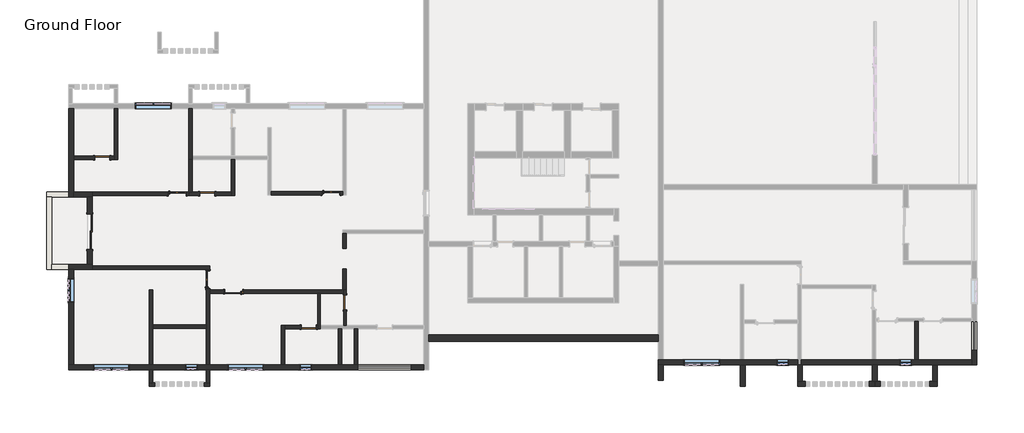
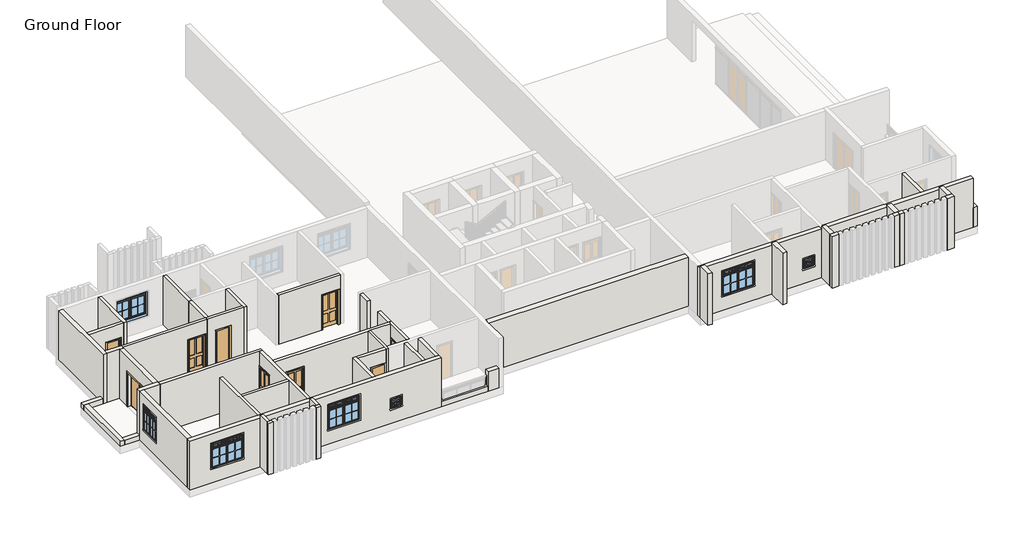
# One storey, part 1 of 9: 51 walls, 9 doors, 9 windows.
# Revit data of these elements (continued)
# Elements 43, 44 (IfcWall, "9\" EXTERIOR WALL")
#   Top Offset = 0' - 0"
#   Base Offset = 0' - 0"
#   Unconnected Height = 1' - 0"
#   wall height = 1' - 0"
#   Phase Created = New Construction
#   Base Constraint = Ground Floor
#   Materials on its faces: "0 Cream", "Default Wall"
# Element 46 (IfcWall, "9\" EXTERIOR WALL")
#   Top Offset = 0' - 0"
#   Base Offset = 0' - 0"
#   wall height = 10' - 6"
#   Phase Created = New Construction
#   Base Constraint = Ground Floor
#   Top Constraint = 1st Floor
#   Materials on its faces: "Default Wall", "0 Cream", "0 olive green"
# Element 49 (IfcWall, "9\" EXTERIOR WALL")
#   Top Offset = 0' - 0"
#   Base Offset = 0' - 0"
#   Unconnected Height = 4' - 0"
#   wall height = 4' - 0"
#   Phase Created = New Construction
#   Base Constraint = Ground Floor
#   Materials on its faces: "Default Wall", "0 Cream"
# Element 51 (IfcWall, "9\" EXTERIOR WALL")
#   Top Offset = 0' - 0"
#   Base Offset = 0' - 0"
#   Unconnected Height = 4' - 0"
#   wall height = 4' - 0"
#   Phase Created = New Construction
#   Base Constraint = Ground Floor
#   Materials on its faces: "0 Cream", "Default Wall"
# Element 61 (IfcWindow, "Window-Casement-Double-Awning-Double : 4' x 5' Window")
#   Mark = "28"
#   Window Inset = 0' - 0"
#   Interior Wall Closure = 0' - 2 1/4"
#   Frame Extension = 0' - 0 1/4"
#   Exterior Wall Closure = 0' - 1 1/4"
#   Interior Trim Visibility = yes
#   Exterior Trim Visibility = yes
#   Phase Created = New Construction
#   Materials on its faces: "Wood - Stained", "Glass", "Clad - White"
# Element 62 (IfcWindow, "Window-Casement-Double-Awning-Double : 6' x 5'")
#   Mark = "1"
#   Window Inset = 0' - 0"
#   Interior Wall Closure = 0' - 2 1/4"
#   Frame Extension = 0' - 0 1/4"
#   Exterior Wall Closure = 0' - 1 1/4"
#   Interior Trim Visibility = yes
#   Exterior Trim Visibility = yes
#   Phase Created = New Construction
#   Materials on its faces: "Wood - Stained", "Glass", "Clad - White"
# Element 63 (IfcWindow, "Window-Casement-Double-Awning-Double : 6' x 5'")
#   Mark = "2"
#   Window Inset = 0' - 0"
#   Interior Wall Closure = 0' - 2 1/4"
#   Frame Extension = 0' - 0 1/4"
#   Exterior Wall Closure = 0' - 1 1/4"
#   Interior Trim Visibility = yes
#   Exterior Trim Visibility = yes
#   Phase Created = New Construction
#   Materials on its faces: "Wood - Stained", "Glass", "Clad - White"
# Element 64 (IfcWindow, "Window-Casement-Double-Awning-Double : 6' x 5'")
#   Mark = "4"
#   Window Inset = 0' - 0"
#   Interior Wall Closure = 0' - 2 1/4"
#   Frame Extension = 0' - 0 1/4"
#   Exterior Wall Closure = 0' - 1 1/4"
#   Interior Trim Visibility = yes
#   Exterior Trim Visibility = yes
#   Phase Created = New Construction
#   Materials on its faces: "Wood - Stained", "Glass", "Clad - White"
# Element 65 (IfcWindow, "Window-Casement-Double-Awning-Double : 6' x 5'")
#   Mark = "20"
#   Window Inset = 0' - 0"
#   Interior Wall Closure = 0' - 2 1/4"
#   Frame Extension = 0' - 0 1/4"
#   Exterior Wall Closure = 0' - 1 1/4"
#   Interior Trim Visibility = yes
#   Exterior Trim Visibility = yes
#   Phase Created = New Construction
#   Materials on its faces: "Wood - Stained", "Glass", "Clad - White"
# Element 66 (IfcWindow, "Window-Double-Hung")
#   Mark = "18"
#   Window Inset = 0' - 0"
#   Interior Wall Closure = 0' - 1 1/2"
#   Frame Extension = 0' - 1 1/4"
#   Exterior Wall Closure = 0' - 0 1/2"
#   Interior Trim Visibility = yes
#   Indicator Visibility = yes
#   Exterior Trim Visibility = yes
#   Phase Created = New Construction
#   Materials on its faces: "Wood - Stained", "Glass", "Clad - White"
# Element 67 (IfcWindow, "Window-Double-Hung")
#   Mark = "19"
#   Window Inset = 0' - 0"
#   Interior Wall Closure = 0' - 1 1/2"
#   Frame Extension = 0' - 1 1/4"
#   Exterior Wall Closure = 0' - 0 1/2"
#   Interior Trim Visibility = yes
#   Indicator Visibility = yes
#   Exterior Trim Visibility = yes
#   Phase Created = New Construction
#   Materials on its faces: "Wood - Stained", "Glass", "Clad - White"
# Element 68 (IfcWindow, "Window-Double-Hung")
#   Mark = "26"
#   Window Inset = 0' - 0"
#   Interior Wall Closure = 0' - 1 1/2"
#   Frame Extension = 0' - 1 1/4"
#   Exterior Wall Closure = 0' - 0 1/2"
#   Interior Trim Visibility = yes
#   Indicator Visibility = yes
#   Exterior Trim Visibility = yes
#   Phase Created = New Construction
#   Materials on its faces: "Wood - Stained", "Glass", "Clad - White"
# Element 69 (IfcWindow, "Window-Double-Hung")
#   Mark = "27"
#   Window Inset = 0' - 0"
#   Interior Wall Closure = 0' - 1 1/2"
#   Frame Extension = 0' - 1 1/4"
#   Exterior Wall Closure = 0' - 0 1/2"
#   Interior Trim Visibility = yes
#   Indicator Visibility = yes
#   Exterior Trim Visibility = yes
#   Phase Created = New Construction
#   Materials on its faces: "Wood - Stained", "Glass", "Clad - White"
# Materials
#   "Glass": class "Glass", colour RGB 0 128 192, transparency 0.75, Description = "Soda Lime Glass", Cost = 0
#   "Wood - Birch - Solid Stained Light Low Gloss": class "Wood", colour RGB 210 159 95, transparency 0, Cost = 0
#   "Paint - Sienna": colour RGB 118 70 51, transparency 0, Cost = 0
#   "Cherry": class "Wood", colour RGB 226 177 128, transparency 0, Description = "Prunus Serotina", Cost = 0
#   "Aluminum": class "Metal", colour RGB 247 247 247, transparency 0, Description = "Aluminum 6061", Cost = 0
#   "Door - Panel": class "Wood", colour RGB 210 159 95, transparency 0, Cost = 0
#   "Door - Frame": colour RGB 118 70 51, transparency 0, Cost = 0
#   "0 Cream": class "Generic", colour RGB 120 120 120, transparency 0, Cost = 0
#   "Wood - Stained": class "Wood", colour RGB 224 178 126, transparency 0, Cost = 0
#   "Clad - White": class "Wood", colour RGB 242 242 238, transparency 0, Cost = 0
#   "Default Wall": colour RGB 128 128 128, transparency 0, Cost = 0
#   "0 olive green": class "Generic", colour RGB 120 120 120, transparency 0, Cost = 0
